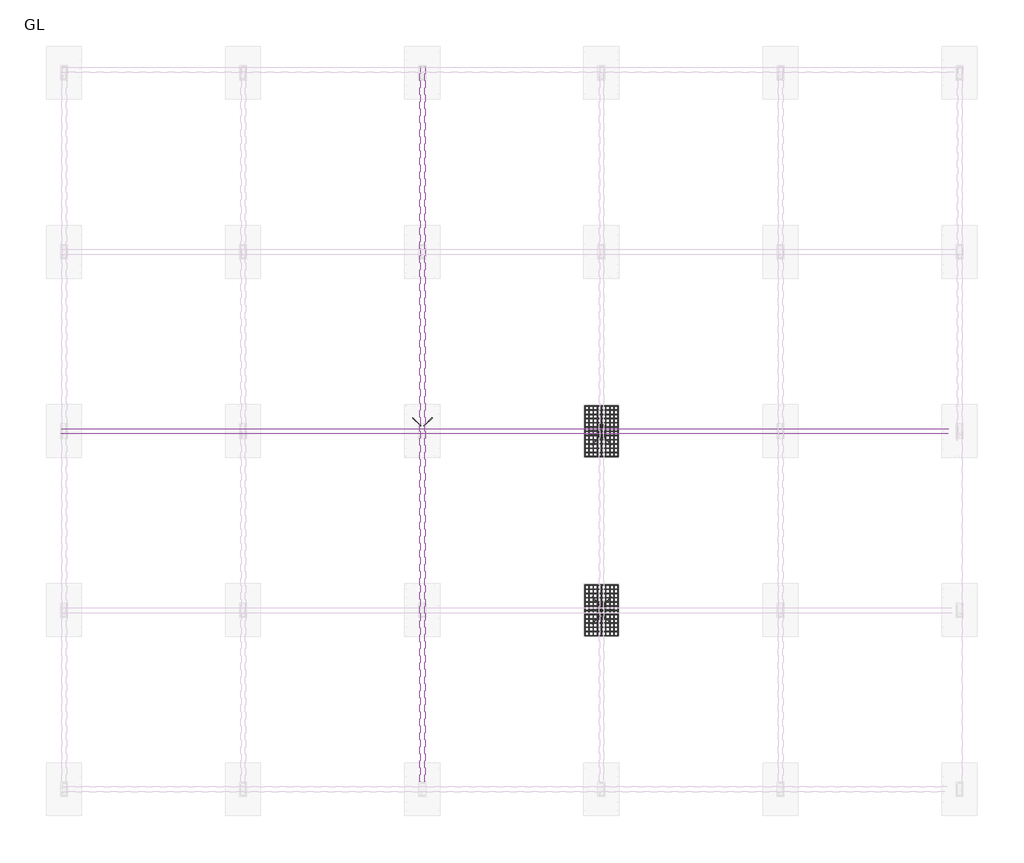
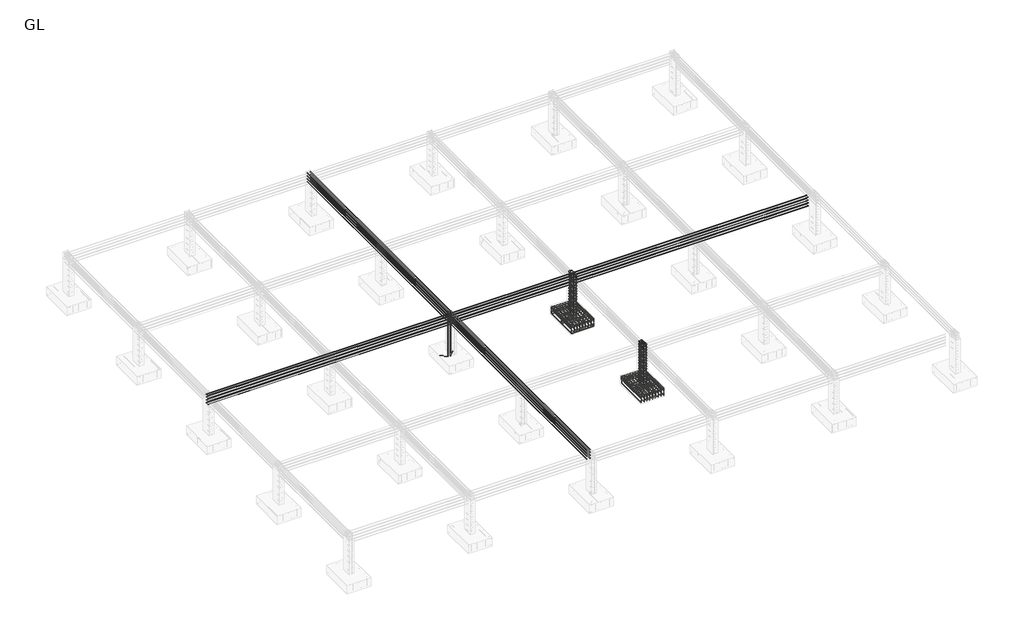
# One storey, part 8 of 16: 24 reinforcing bars.
"""IFC4 building model written with IfcOpenShell, lengths in millimetres."""

from ifc_helpers import new_model, si_unit, point, frame, origin, place, context, project, spatial, polyline, circle_curve, trimmed, segment, composite_curve, source, transform, mapped, element, save
from ifc_brep_helpers import swept_disk

model = new_model("IFC4")

# Units and contexts
model_context = context("Model", 3, world=origin())
ifc_project = project(units=[si_unit("LENGTHUNIT", "METRE", prefix="MILLI")], contexts=[model_context])

# Site, building, storey
site = spatial("IfcSite", under=ifc_project)
building = spatial("IfcBuilding", under=site)
storey = spatial("IfcBuildingStorey", under=building, Name="GL", Elevation=-1829.0)

# Reinforcing bars
placement = place(None, origin())
reinforcing_bar_shape = source(origin(), model_context, "Body", "SolidModel", [
    swept_disk(composite_curve([segment(polyline([(-3954.9544379, -7223.1167521, -2089.0), (-3954.9544379, -7223.1167521, -2213.0)]), True, "CONTINUOUS"), segment(trimmed(circle_curve(frame((-3984.9544379, -7223.1167521, -2213.0), z_axis=(0.0, 1.0, 0.0), x_axis=(30.0, 0.0, 0.0)), 30.0), [point((-3954.9544379, -7223.1167521, -2213.0))], [point((-3984.9544379, -7223.1167521, -2243.0))], True, "CARTESIAN"), True, "CONTINUOUS"), segment(polyline([(-3984.9544379, -7223.1167521, -2243.0), (-5052.9544379, -7223.1167521, -2243.0)]), True, "CONTINUOUS"), segment(trimmed(circle_curve(frame((-5052.9544379, -7223.1167521, -2213.0), z_axis=(0.0, 1.0, 0.0), x_axis=(0.0, 0.0, -30.0)), 30.0), [point((-5052.9544379, -7223.1167521, -2243.0))], [point((-5082.9544379, -7223.1167521, -2213.0))], True, "CARTESIAN"), True, "CONTINUOUS"), segment(polyline([(-5082.9544379, -7223.1167521, -2213.0), (-5082.9544379, -7223.1167521, -2089.0)]), True, "CONTINUOUS")], self_intersect=False), 6.0),
])
element("IfcReinforcingBar", 1, at=placement, inside=storey, context=model_context, shape_type="MappedRepresentation", body=[
    mapped(reinforcing_bar_shape, transform((0.0, 0.0, 0.0), x_axis=(1.0, 0.0, 0.0), y_axis=(0.0, 1.0, 0.0), z_axis=(0.0, 0.0, 1.0))),
    mapped(reinforcing_bar_shape, transform((0.0, -864.0, 0.0), x_axis=(1.0, 0.0, 0.0), y_axis=(0.0, 1.0, 0.0), z_axis=(0.0, 0.0, 1.0))),
    mapped(reinforcing_bar_shape, transform((0.0, -1728.0, 0.0), x_axis=(1.0, 0.0, 0.0), y_axis=(0.0, 1.0, 0.0), z_axis=(0.0, 0.0, 1.0))),
])
reinforcing_bar_2_shape = source(origin(), model_context, "Body", "SolidModel", [
    swept_disk(composite_curve([segment(polyline([(-5082.9544379, -7223.1167521, -2022.436678), (-5082.9544379, -7223.1167521, -1898.436678)]), True, "CONTINUOUS"), segment(trimmed(circle_curve(frame((-5052.9544379, -7223.1167521, -1898.436678), z_axis=(0.0, 1.0, 0.0), x_axis=(-30.0, 0.0, 0.0)), 30.0), [point((-5082.9544379, -7223.1167521, -1898.436678))], [point((-5052.9544379, -7223.1167521, -1868.436678))], True, "CARTESIAN"), True, "CONTINUOUS"), segment(polyline([(-5052.9544379, -7223.1167521, -1868.436678), (-3984.9544379, -7223.1167521, -1868.436678)]), True, "CONTINUOUS"), segment(trimmed(circle_curve(frame((-3984.9544379, -7223.1167521, -1898.436678), z_axis=(0.0, 1.0, 0.0), x_axis=(0.0, 0.0, 30.0)), 30.0), [point((-3984.9544379, -7223.1167521, -1868.436678))], [point((-3954.9544379, -7223.1167521, -1898.436678))], True, "CARTESIAN"), True, "CONTINUOUS"), segment(polyline([(-3954.9544379, -7223.1167521, -1898.436678), (-3954.9544379, -7223.1167521, -2022.436678)]), True, "CONTINUOUS")], self_intersect=False), 6.0),
])
element("IfcReinforcingBar", 2, at=placement, inside=storey, context=model_context, shape_type="MappedRepresentation", body=[
    mapped(reinforcing_bar_2_shape, transform((0.0, 0.0, 0.0), x_axis=(1.0, 0.0, 0.0), y_axis=(0.0, 1.0, 0.0), z_axis=(0.0, 0.0, 1.0))),
    mapped(reinforcing_bar_2_shape, transform((0.0, -144.0, 0.0), x_axis=(1.0, 0.0, 0.0), y_axis=(0.0, 1.0, 0.0), z_axis=(0.0, 0.0, 1.0))),
    mapped(reinforcing_bar_2_shape, transform((0.0, -288.0, 0.0), x_axis=(1.0, 0.0, 0.0), y_axis=(0.0, 1.0, 0.0), z_axis=(0.0, 0.0, 1.0))),
    mapped(reinforcing_bar_2_shape, transform((0.0, -432.0, 0.0), x_axis=(1.0, 0.0, 0.0), y_axis=(0.0, 1.0, 0.0), z_axis=(0.0, 0.0, 1.0))),
    mapped(reinforcing_bar_2_shape, transform((0.0, -576.0, 0.0), x_axis=(1.0, 0.0, 0.0), y_axis=(0.0, 1.0, 0.0), z_axis=(0.0, 0.0, 1.0))),
    mapped(reinforcing_bar_2_shape, transform((0.0, -720.0, 0.0), x_axis=(1.0, 0.0, 0.0), y_axis=(0.0, 1.0, 0.0), z_axis=(0.0, 0.0, 1.0))),
    mapped(reinforcing_bar_2_shape, transform((0.0, -864.0, 0.0), x_axis=(1.0, 0.0, 0.0), y_axis=(0.0, 1.0, 0.0), z_axis=(0.0, 0.0, 1.0))),
    mapped(reinforcing_bar_2_shape, transform((0.0, -1008.0, 0.0), x_axis=(1.0, 0.0, 0.0), y_axis=(0.0, 1.0, 0.0), z_axis=(0.0, 0.0, 1.0))),
    mapped(reinforcing_bar_2_shape, transform((0.0, -1152.0, 0.0), x_axis=(1.0, 0.0, 0.0), y_axis=(0.0, 1.0, 0.0), z_axis=(0.0, 0.0, 1.0))),
    mapped(reinforcing_bar_2_shape, transform((0.0, -1296.0, 0.0), x_axis=(1.0, 0.0, 0.0), y_axis=(0.0, 1.0, 0.0), z_axis=(0.0, 0.0, 1.0))),
    mapped(reinforcing_bar_2_shape, transform((0.0, -1440.0, 0.0), x_axis=(1.0, 0.0, 0.0), y_axis=(0.0, 1.0, 0.0), z_axis=(0.0, 0.0, 1.0))),
    mapped(reinforcing_bar_2_shape, transform((0.0, -1584.0, 0.0), x_axis=(1.0, 0.0, 0.0), y_axis=(0.0, 1.0, 0.0), z_axis=(0.0, 0.0, 1.0))),
    mapped(reinforcing_bar_2_shape, transform((0.0, -1728.0, 0.0), x_axis=(1.0, 0.0, 0.0), y_axis=(0.0, 1.0, 0.0), z_axis=(0.0, 0.0, 1.0))),
])
reinforcing_bar_3_shape = source(origin(), model_context, "Body", "SolidModel", [
    swept_disk(composite_curve([segment(polyline([(-5082.9544379, -8951.1167521, -2027.5081232), (-5082.9544379, -8951.1167521, -1903.5081232)]), True, "CONTINUOUS"), segment(trimmed(circle_curve(frame((-5082.9544379, -8921.1167521, -1903.5081232), z_axis=(-1.0, 0.0, 0.0), x_axis=(0.0, -30.0, 0.0)), 30.0), [point((-5082.9544379, -8951.1167521, -1903.5081232))], [point((-5082.9544379, -8921.1167521, -1873.5081232))], True, "CARTESIAN"), True, "CONTINUOUS"), segment(polyline([(-5082.9544379, -8921.1167521, -1873.5081232), (-5082.9544379, -7253.1167521, -1873.5081232)]), True, "CONTINUOUS"), segment(trimmed(circle_curve(frame((-5082.9544379, -7253.1167521, -1903.5081232), z_axis=(-1.0, 0.0, 0.0), x_axis=(0.0, 0.0, 30.0)), 30.0), [point((-5082.9544379, -7253.1167521, -1873.5081232))], [point((-5082.9544379, -7223.1167521, -1903.5081232))], True, "CARTESIAN"), True, "CONTINUOUS"), segment(polyline([(-5082.9544379, -7223.1167521, -1903.5081232), (-5082.9544379, -7223.1167521, -2027.5081232)]), True, "CONTINUOUS")], self_intersect=False), 6.0),
])
element("IfcReinforcingBar", 3, at=placement, inside=storey, context=model_context, shape_type="MappedRepresentation", body=[
    mapped(reinforcing_bar_3_shape, transform((0.0, 0.0, 0.0), x_axis=(1.0, 0.0, 0.0), y_axis=(0.0, 1.0, 0.0), z_axis=(0.0, 0.0, 1.0))),
    mapped(reinforcing_bar_3_shape, transform((141.0, 0.0, 0.0), x_axis=(1.0, 0.0, 0.0), y_axis=(0.0, 1.0, 0.0), z_axis=(0.0, 0.0, 1.0))),
    mapped(reinforcing_bar_3_shape, transform((282.0, 0.0, 0.0), x_axis=(1.0, 0.0, 0.0), y_axis=(0.0, 1.0, 0.0), z_axis=(0.0, 0.0, 1.0))),
    mapped(reinforcing_bar_3_shape, transform((423.0, 0.0, 0.0), x_axis=(1.0, 0.0, 0.0), y_axis=(0.0, 1.0, 0.0), z_axis=(0.0, 0.0, 1.0))),
    mapped(reinforcing_bar_3_shape, transform((564.0, 0.0, 0.0), x_axis=(1.0, 0.0, 0.0), y_axis=(0.0, 1.0, 0.0), z_axis=(0.0, 0.0, 1.0))),
    mapped(reinforcing_bar_3_shape, transform((705.0, 0.0, 0.0), x_axis=(1.0, 0.0, 0.0), y_axis=(0.0, 1.0, 0.0), z_axis=(0.0, 0.0, 1.0))),
    mapped(reinforcing_bar_3_shape, transform((846.0, 0.0, 0.0), x_axis=(1.0, 0.0, 0.0), y_axis=(0.0, 1.0, 0.0), z_axis=(0.0, 0.0, 1.0))),
    mapped(reinforcing_bar_3_shape, transform((987.0, 0.0, 0.0), x_axis=(1.0, 0.0, 0.0), y_axis=(0.0, 1.0, 0.0), z_axis=(0.0, 0.0, 1.0))),
    mapped(reinforcing_bar_3_shape, transform((1128.0, 0.0, 0.0), x_axis=(1.0, 0.0, 0.0), y_axis=(0.0, 1.0, 0.0), z_axis=(0.0, 0.0, 1.0))),
])
reinforcing_bar_4_shape = source(origin(), model_context, "Body", "SolidModel", [
    swept_disk(composite_curve([segment(polyline([(-3954.9544379, -8951.1167521, -2080.6239909), (-3954.9544379, -8951.1167521, -2204.6239909)]), True, "CONTINUOUS"), segment(trimmed(circle_curve(frame((-3954.9544379, -8921.1167521, -2204.6239909), z_axis=(1.0, 0.0, 0.0), x_axis=(0.0, -30.0, 0.0)), 30.0), [point((-3954.9544379, -8951.1167521, -2204.6239909))], [point((-3954.9544379, -8921.1167521, -2234.6239909))], True, "CARTESIAN"), True, "CONTINUOUS"), segment(polyline([(-3954.9544379, -8921.1167521, -2234.6239909), (-3954.9544379, -7266.1421892, -2234.6239909)]), True, "CONTINUOUS"), segment(trimmed(circle_curve(frame((-3954.9544379, -7266.1421892, -2204.6239909), z_axis=(1.0, 0.0, 0.0), x_axis=(0.0, 0.0, -30.0)), 30.0), [point((-3954.9544379, -7266.1421892, -2234.6239909))], [point((-3954.9544379, -7236.1421892, -2204.6239909))], True, "CARTESIAN"), True, "CONTINUOUS"), segment(polyline([(-3954.9544379, -7236.1421892, -2204.6239909), (-3954.9544379, -7236.1421892, -2080.6239909)]), True, "CONTINUOUS")], self_intersect=False), 6.0),
])
element("IfcReinforcingBar", 4, at=placement, inside=storey, context=model_context, shape_type="MappedRepresentation", body=[
    mapped(reinforcing_bar_4_shape, transform((0.0, 0.0, 0.0), x_axis=(1.0, 0.0, 0.0), y_axis=(0.0, 1.0, 0.0), z_axis=(0.0, 0.0, 1.0))),
    mapped(reinforcing_bar_4_shape, transform((-141.0, 0.0, 0.0), x_axis=(1.0, 0.0, 0.0), y_axis=(0.0, 1.0, 0.0), z_axis=(0.0, 0.0, 1.0))),
    mapped(reinforcing_bar_4_shape, transform((-282.0, 0.0, 0.0), x_axis=(1.0, 0.0, 0.0), y_axis=(0.0, 1.0, 0.0), z_axis=(0.0, 0.0, 1.0))),
    mapped(reinforcing_bar_4_shape, transform((-423.0, 0.0, 0.0), x_axis=(1.0, 0.0, 0.0), y_axis=(0.0, 1.0, 0.0), z_axis=(0.0, 0.0, 1.0))),
    mapped(reinforcing_bar_4_shape, transform((-564.0, 0.0, 0.0), x_axis=(1.0, 0.0, 0.0), y_axis=(0.0, 1.0, 0.0), z_axis=(0.0, 0.0, 1.0))),
    mapped(reinforcing_bar_4_shape, transform((-705.0, 0.0, 0.0), x_axis=(1.0, 0.0, 0.0), y_axis=(0.0, 1.0, 0.0), z_axis=(0.0, 0.0, 1.0))),
    mapped(reinforcing_bar_4_shape, transform((-846.0, 0.0, 0.0), x_axis=(1.0, 0.0, 0.0), y_axis=(0.0, 1.0, 0.0), z_axis=(0.0, 0.0, 1.0))),
    mapped(reinforcing_bar_4_shape, transform((-987.0, 0.0, 0.0), x_axis=(1.0, 0.0, 0.0), y_axis=(0.0, 1.0, 0.0), z_axis=(0.0, 0.0, 1.0))),
    mapped(reinforcing_bar_4_shape, transform((-1128.0, 0.0, 0.0), x_axis=(1.0, 0.0, 0.0), y_axis=(0.0, 1.0, 0.0), z_axis=(0.0, 0.0, 1.0))),
])
reinforcing_bar_5_shape = source(origin(), model_context, "Body", "SolidModel", [
    swept_disk(composite_curve([segment(polyline([(-5082.9544379, -13319.1167521, -2022.436678), (-5082.9544379, -13319.1167521, -1898.436678)]), True, "CONTINUOUS"), segment(trimmed(circle_curve(frame((-5052.9544379, -13319.1167521, -1898.436678), z_axis=(0.0, 1.0, 0.0), x_axis=(-30.0, 0.0, 0.0)), 30.0), [point((-5082.9544379, -13319.1167521, -1898.436678))], [point((-5052.9544379, -13319.1167521, -1868.436678))], True, "CARTESIAN"), True, "CONTINUOUS"), segment(polyline([(-5052.9544379, -13319.1167521, -1868.436678), (-3984.9544379, -13319.1167521, -1868.436678)]), True, "CONTINUOUS"), segment(trimmed(circle_curve(frame((-3984.9544379, -13319.1167521, -1898.436678), z_axis=(0.0, 1.0, 0.0), x_axis=(0.0, 0.0, 30.0)), 30.0), [point((-3984.9544379, -13319.1167521, -1868.436678))], [point((-3954.9544379, -13319.1167521, -1898.436678))], True, "CARTESIAN"), True, "CONTINUOUS"), segment(polyline([(-3954.9544379, -13319.1167521, -1898.436678), (-3954.9544379, -13319.1167521, -2022.436678)]), True, "CONTINUOUS")], self_intersect=False), 6.0),
])
element("IfcReinforcingBar", 5, at=placement, inside=storey, context=model_context, shape_type="MappedRepresentation", body=[
    mapped(reinforcing_bar_5_shape, transform((0.0, 0.0, 0.0), x_axis=(1.0, 0.0, 0.0), y_axis=(0.0, 1.0, 0.0), z_axis=(0.0, 0.0, 1.0))),
    mapped(reinforcing_bar_5_shape, transform((0.0, -144.0, 0.0), x_axis=(1.0, 0.0, 0.0), y_axis=(0.0, 1.0, 0.0), z_axis=(0.0, 0.0, 1.0))),
    mapped(reinforcing_bar_5_shape, transform((0.0, -288.0, 0.0), x_axis=(1.0, 0.0, 0.0), y_axis=(0.0, 1.0, 0.0), z_axis=(0.0, 0.0, 1.0))),
    mapped(reinforcing_bar_5_shape, transform((0.0, -432.0, 0.0), x_axis=(1.0, 0.0, 0.0), y_axis=(0.0, 1.0, 0.0), z_axis=(0.0, 0.0, 1.0))),
    mapped(reinforcing_bar_5_shape, transform((0.0, -576.0, 0.0), x_axis=(1.0, 0.0, 0.0), y_axis=(0.0, 1.0, 0.0), z_axis=(0.0, 0.0, 1.0))),
    mapped(reinforcing_bar_5_shape, transform((0.0, -720.0, 0.0), x_axis=(1.0, 0.0, 0.0), y_axis=(0.0, 1.0, 0.0), z_axis=(0.0, 0.0, 1.0))),
    mapped(reinforcing_bar_5_shape, transform((0.0, -864.0, 0.0), x_axis=(1.0, 0.0, 0.0), y_axis=(0.0, 1.0, 0.0), z_axis=(0.0, 0.0, 1.0))),
    mapped(reinforcing_bar_5_shape, transform((0.0, -1008.0, 0.0), x_axis=(1.0, 0.0, 0.0), y_axis=(0.0, 1.0, 0.0), z_axis=(0.0, 0.0, 1.0))),
    mapped(reinforcing_bar_5_shape, transform((0.0, -1152.0, 0.0), x_axis=(1.0, 0.0, 0.0), y_axis=(0.0, 1.0, 0.0), z_axis=(0.0, 0.0, 1.0))),
    mapped(reinforcing_bar_5_shape, transform((0.0, -1296.0, 0.0), x_axis=(1.0, 0.0, 0.0), y_axis=(0.0, 1.0, 0.0), z_axis=(0.0, 0.0, 1.0))),
    mapped(reinforcing_bar_5_shape, transform((0.0, -1440.0, 0.0), x_axis=(1.0, 0.0, 0.0), y_axis=(0.0, 1.0, 0.0), z_axis=(0.0, 0.0, 1.0))),
    mapped(reinforcing_bar_5_shape, transform((0.0, -1584.0, 0.0), x_axis=(1.0, 0.0, 0.0), y_axis=(0.0, 1.0, 0.0), z_axis=(0.0, 0.0, 1.0))),
    mapped(reinforcing_bar_5_shape, transform((0.0, -1728.0, 0.0), x_axis=(1.0, 0.0, 0.0), y_axis=(0.0, 1.0, 0.0), z_axis=(0.0, 0.0, 1.0))),
])
reinforcing_bar_6_shape = source(origin(), model_context, "Body", "SolidModel", [
    swept_disk(composite_curve([segment(polyline([(-5082.9544379, -15047.1167521, -2027.5081232), (-5082.9544379, -15047.1167521, -1903.5081232)]), True, "CONTINUOUS"), segment(trimmed(circle_curve(frame((-5082.9544379, -15017.1167521, -1903.5081232), z_axis=(-1.0, 0.0, 0.0), x_axis=(0.0, -30.0, 0.0)), 30.0), [point((-5082.9544379, -15047.1167521, -1903.5081232))], [point((-5082.9544379, -15017.1167521, -1873.5081232))], True, "CARTESIAN"), True, "CONTINUOUS"), segment(polyline([(-5082.9544379, -15017.1167521, -1873.5081232), (-5082.9544379, -13349.1167521, -1873.5081232)]), True, "CONTINUOUS"), segment(trimmed(circle_curve(frame((-5082.9544379, -13349.1167521, -1903.5081232), z_axis=(-1.0, 0.0, 0.0), x_axis=(0.0, 0.0, 30.0)), 30.0), [point((-5082.9544379, -13349.1167521, -1873.5081232))], [point((-5082.9544379, -13319.1167521, -1903.5081232))], True, "CARTESIAN"), True, "CONTINUOUS"), segment(polyline([(-5082.9544379, -13319.1167521, -1903.5081232), (-5082.9544379, -13319.1167521, -2027.5081232)]), True, "CONTINUOUS")], self_intersect=False), 6.0),
])
element("IfcReinforcingBar", 6, at=placement, inside=storey, context=model_context, shape_type="MappedRepresentation", body=[
    mapped(reinforcing_bar_6_shape, transform((0.0, 0.0, 0.0), x_axis=(1.0, 0.0, 0.0), y_axis=(0.0, 1.0, 0.0), z_axis=(0.0, 0.0, 1.0))),
    mapped(reinforcing_bar_6_shape, transform((141.0, 0.0, 0.0), x_axis=(1.0, 0.0, 0.0), y_axis=(0.0, 1.0, 0.0), z_axis=(0.0, 0.0, 1.0))),
    mapped(reinforcing_bar_6_shape, transform((282.0, 0.0, 0.0), x_axis=(1.0, 0.0, 0.0), y_axis=(0.0, 1.0, 0.0), z_axis=(0.0, 0.0, 1.0))),
    mapped(reinforcing_bar_6_shape, transform((423.0, 0.0, 0.0), x_axis=(1.0, 0.0, 0.0), y_axis=(0.0, 1.0, 0.0), z_axis=(0.0, 0.0, 1.0))),
    mapped(reinforcing_bar_6_shape, transform((564.0, 0.0, 0.0), x_axis=(1.0, 0.0, 0.0), y_axis=(0.0, 1.0, 0.0), z_axis=(0.0, 0.0, 1.0))),
    mapped(reinforcing_bar_6_shape, transform((705.0, 0.0, 0.0), x_axis=(1.0, 0.0, 0.0), y_axis=(0.0, 1.0, 0.0), z_axis=(0.0, 0.0, 1.0))),
    mapped(reinforcing_bar_6_shape, transform((846.0, 0.0, 0.0), x_axis=(1.0, 0.0, 0.0), y_axis=(0.0, 1.0, 0.0), z_axis=(0.0, 0.0, 1.0))),
    mapped(reinforcing_bar_6_shape, transform((987.0, 0.0, 0.0), x_axis=(1.0, 0.0, 0.0), y_axis=(0.0, 1.0, 0.0), z_axis=(0.0, 0.0, 1.0))),
    mapped(reinforcing_bar_6_shape, transform((1128.0, 0.0, 0.0), x_axis=(1.0, 0.0, 0.0), y_axis=(0.0, 1.0, 0.0), z_axis=(0.0, 0.0, 1.0))),
])
reinforcing_bar_7_shape = source(origin(), model_context, "Body", "SolidModel", [
    swept_disk(composite_curve([segment(polyline([(-3954.9544379, -15047.1167521, -2080.6239909), (-3954.9544379, -15047.1167521, -2204.6239909)]), True, "CONTINUOUS"), segment(trimmed(circle_curve(frame((-3954.9544379, -15017.1167521, -2204.6239909), z_axis=(1.0, 0.0, 0.0), x_axis=(0.0, -30.0, 0.0)), 30.0), [point((-3954.9544379, -15047.1167521, -2204.6239909))], [point((-3954.9544379, -15017.1167521, -2234.6239909))], True, "CARTESIAN"), True, "CONTINUOUS"), segment(polyline([(-3954.9544379, -15017.1167521, -2234.6239909), (-3954.9544379, -13362.1421892, -2234.6239909)]), True, "CONTINUOUS"), segment(trimmed(circle_curve(frame((-3954.9544379, -13362.1421892, -2204.6239909), z_axis=(1.0, 0.0, 0.0), x_axis=(0.0, 0.0, -30.0)), 30.0), [point((-3954.9544379, -13362.1421892, -2234.6239909))], [point((-3954.9544379, -13332.1421892, -2204.6239909))], True, "CARTESIAN"), True, "CONTINUOUS"), segment(polyline([(-3954.9544379, -13332.1421892, -2204.6239909), (-3954.9544379, -13332.1421892, -2080.6239909)]), True, "CONTINUOUS")], self_intersect=False), 6.0),
])
element("IfcReinforcingBar", 7, at=placement, inside=storey, context=model_context, shape_type="MappedRepresentation", body=[
    mapped(reinforcing_bar_7_shape, transform((0.0, 0.0, 0.0), x_axis=(1.0, 0.0, 0.0), y_axis=(0.0, 1.0, 0.0), z_axis=(0.0, 0.0, 1.0))),
    mapped(reinforcing_bar_7_shape, transform((-141.0, 0.0, 0.0), x_axis=(1.0, 0.0, 0.0), y_axis=(0.0, 1.0, 0.0), z_axis=(0.0, 0.0, 1.0))),
    mapped(reinforcing_bar_7_shape, transform((-282.0, 0.0, 0.0), x_axis=(1.0, 0.0, 0.0), y_axis=(0.0, 1.0, 0.0), z_axis=(0.0, 0.0, 1.0))),
    mapped(reinforcing_bar_7_shape, transform((-423.0, 0.0, 0.0), x_axis=(1.0, 0.0, 0.0), y_axis=(0.0, 1.0, 0.0), z_axis=(0.0, 0.0, 1.0))),
    mapped(reinforcing_bar_7_shape, transform((-564.0, 0.0, 0.0), x_axis=(1.0, 0.0, 0.0), y_axis=(0.0, 1.0, 0.0), z_axis=(0.0, 0.0, 1.0))),
    mapped(reinforcing_bar_7_shape, transform((-705.0, 0.0, 0.0), x_axis=(1.0, 0.0, 0.0), y_axis=(0.0, 1.0, 0.0), z_axis=(0.0, 0.0, 1.0))),
    mapped(reinforcing_bar_7_shape, transform((-846.0, 0.0, 0.0), x_axis=(1.0, 0.0, 0.0), y_axis=(0.0, 1.0, 0.0), z_axis=(0.0, 0.0, 1.0))),
    mapped(reinforcing_bar_7_shape, transform((-987.0, 0.0, 0.0), x_axis=(1.0, 0.0, 0.0), y_axis=(0.0, 1.0, 0.0), z_axis=(0.0, 0.0, 1.0))),
    mapped(reinforcing_bar_7_shape, transform((-1128.0, 0.0, 0.0), x_axis=(1.0, 0.0, 0.0), y_axis=(0.0, 1.0, 0.0), z_axis=(0.0, 0.0, 1.0))),
])
element("IfcReinforcingBar", 8, at=placement, inside=storey, context=model_context, shape_type="SolidModel", body=[
    swept_disk(composite_curve([segment(polyline([(-10672.0642232, -7902.1692603, 241.0), (-10672.0642232, -7902.1692603, -2129.0)]), True, "CONTINUOUS"), segment(trimmed(circle_curve(frame((-10693.2774266, -7880.9560568, -2129.0), z_axis=(0.7071067811865218, 0.7071067811865733, 0.0), x_axis=(21.213203400000566, -21.213203500000418, 0.0)), 30.0), [point((-10672.0642232, -7902.1692603, -2129.0))], [point((-10693.2774266, -7880.9560568, -2159.0))], True, "CARTESIAN"), True, "CONTINUOUS"), segment(polyline([(-10693.2774266, -7880.9560568, -2159.0), (-10940.7648, -7633.4686834, -2159.0)]), True, "CONTINUOUS")], self_intersect=False), 6.0),
])
element("IfcReinforcingBar", 9, at=placement, inside=storey, context=model_context, shape_type="SolidModel", body=[
    swept_disk(composite_curve([segment(polyline([(-10557.8446527, -7902.1692603, 241.0), (-10557.8446527, -7902.1692603, -2129.0)]), True, "CONTINUOUS"), segment(trimmed(circle_curve(frame((-10536.6314492, -7880.9560568, -2129.0), z_axis=(0.7071067811865157, -0.7071067811865794, 0.0), x_axis=(-21.21320349999951, -21.213203500000418, 0.0)), 30.0), [point((-10557.8446527, -7902.1692603, -2129.0))], [point((-10536.6314492, -7880.9560568, -2159.0))], True, "CARTESIAN"), True, "CONTINUOUS"), segment(polyline([(-10536.6314492, -7880.9560568, -2159.0), (-10289.1440758, -7633.4686834, -2159.0)]), True, "CONTINUOUS")], self_intersect=False), 6.0),
])
reinforcing_bar_8_shape = source(origin(), model_context, "Body", "SolidModel", [
    swept_disk(composite_curve([segment(polyline([(-4511.4864005, -8162.2223078, -1793.0), (-4599.1676414, -8249.9035486, -1793.0)]), True, "CONTINUOUS"), segment(trimmed(circle_curve(frame((-4577.9544379, -8271.1167521, -1793.0), z_axis=(0.0, 0.0, 1.0), x_axis=(-21.213203500000418, 21.213203500001327, 0.0)), 30.0), [point((-4599.1676414, -8249.9035486, -1793.0))], [point((-4577.9544379, -8301.1167521, -1793.0))], True, "CARTESIAN"), True, "CONTINUOUS"), segment(polyline([(-4577.9544379, -8301.1167521, -1793.0), (-4459.9544379, -8301.1167521, -1793.0)]), True, "CONTINUOUS"), segment(trimmed(circle_curve(frame((-4459.9544379, -8271.1167521, -1793.0), z_axis=(0.0, 0.0, 1.0), x_axis=(0.0, -30.0, 0.0)), 30.0), [point((-4459.9544379, -8301.1167521, -1793.0))], [point((-4429.9544379, -8271.1167521, -1793.0))], True, "CARTESIAN"), True, "CONTINUOUS"), segment(polyline([(-4429.9544379, -8271.1167521, -1793.0), (-4429.9544379, -7903.1167521, -1793.0)]), True, "CONTINUOUS"), segment(trimmed(circle_curve(frame((-4459.8864962, -7903.1167521, -1795.0178916), z_axis=(-0.06726305234213417, 0.0, 0.9977352764083365), x_axis=(29.93205829999988, 0.0, 2.0178915999999845)), 30.0), [point((-4429.9544379, -7903.1167521, -1793.0))], [point((-4459.8864962, -7873.1167521, -1795.0178916))], True, "CARTESIAN"), True, "CONTINUOUS"), segment(polyline([(-4459.8864962, -7873.1167521, -1795.0178916), (-4578.0223796, -7873.1167521, -1802.9821084)]), True, "CONTINUOUS"), segment(trimmed(circle_curve(frame((-4578.0223796, -7903.1167521, -1802.9821084), z_axis=(-0.06726305234213417, 0.0, 0.9977352764083365), x_axis=(0.0, 30.0, 0.0)), 30.0), [point((-4578.0223796, -7873.1167521, -1802.9821084))], [point((-4607.9544379, -7903.1167521, -1805.0))], True, "CARTESIAN"), True, "CONTINUOUS"), segment(polyline([(-4607.9544379, -7903.1167521, -1805.0), (-4607.9544379, -8271.1167521, -1805.0)]), True, "CONTINUOUS"), segment(trimmed(circle_curve(frame((-4577.9544379, -8271.1167521, -1805.0), z_axis=(0.0, 0.0, 1.0), x_axis=(-30.0, 0.0, 0.0)), 30.0), [point((-4607.9544379, -8271.1167521, -1805.0))], [point((-4556.7412345, -8292.3299555, -1805.0))], True, "CARTESIAN"), True, "CONTINUOUS"), segment(polyline([(-4556.7412345, -8292.3299555, -1805.0), (-4469.0599936, -8204.6487146, -1805.0)]), True, "CONTINUOUS")], self_intersect=False), 6.0),
])
element("IfcReinforcingBar", 10, at=placement, inside=storey, context=model_context, shape_type="MappedRepresentation", body=[
    mapped(reinforcing_bar_8_shape, transform((0.0, 0.0, 0.0), x_axis=(1.0, 0.0, 0.0), y_axis=(0.0, 1.0, 0.0), z_axis=(0.0, 0.0, 1.0))),
    mapped(reinforcing_bar_8_shape, transform((0.0, 0.0, 144.8571429), x_axis=(1.0, 0.0, 0.0), y_axis=(0.0, 1.0, 0.0), z_axis=(0.0, 0.0, 1.0))),
    mapped(reinforcing_bar_8_shape, transform((0.0, 0.0, 289.7142857), x_axis=(1.0, 0.0, 0.0), y_axis=(0.0, 1.0, 0.0), z_axis=(0.0, 0.0, 1.0))),
    mapped(reinforcing_bar_8_shape, transform((0.0, 0.0, 434.5714286), x_axis=(1.0, 0.0, 0.0), y_axis=(0.0, 1.0, 0.0), z_axis=(0.0, 0.0, 1.0))),
    mapped(reinforcing_bar_8_shape, transform((0.0, 0.0, 579.4285714), x_axis=(1.0, 0.0, 0.0), y_axis=(0.0, 1.0, 0.0), z_axis=(0.0, 0.0, 1.0))),
    mapped(reinforcing_bar_8_shape, transform((0.0, 0.0, 724.2857143), x_axis=(1.0, 0.0, 0.0), y_axis=(0.0, 1.0, 0.0), z_axis=(0.0, 0.0, 1.0))),
    mapped(reinforcing_bar_8_shape, transform((0.0, 0.0, 869.1428571), x_axis=(1.0, 0.0, 0.0), y_axis=(0.0, 1.0, 0.0), z_axis=(0.0, 0.0, 1.0))),
    mapped(reinforcing_bar_8_shape, transform((0.0, 0.0, 1014.0), x_axis=(1.0, 0.0, 0.0), y_axis=(0.0, 1.0, 0.0), z_axis=(0.0, 0.0, 1.0))),
    mapped(reinforcing_bar_8_shape, transform((0.0, 0.0, 1158.8571429), x_axis=(1.0, 0.0, 0.0), y_axis=(0.0, 1.0, 0.0), z_axis=(0.0, 0.0, 1.0))),
    mapped(reinforcing_bar_8_shape, transform((0.0, 0.0, 1303.7142857), x_axis=(1.0, 0.0, 0.0), y_axis=(0.0, 1.0, 0.0), z_axis=(0.0, 0.0, 1.0))),
    mapped(reinforcing_bar_8_shape, transform((0.0, 0.0, 1448.5714286), x_axis=(1.0, 0.0, 0.0), y_axis=(0.0, 1.0, 0.0), z_axis=(0.0, 0.0, 1.0))),
    mapped(reinforcing_bar_8_shape, transform((0.0, 0.0, 1593.4285714), x_axis=(1.0, 0.0, 0.0), y_axis=(0.0, 1.0, 0.0), z_axis=(0.0, 0.0, 1.0))),
    mapped(reinforcing_bar_8_shape, transform((0.0, 0.0, 1738.2857143), x_axis=(1.0, 0.0, 0.0), y_axis=(0.0, 1.0, 0.0), z_axis=(0.0, 0.0, 1.0))),
    mapped(reinforcing_bar_8_shape, transform((0.0, 0.0, 1883.1428571), x_axis=(1.0, 0.0, 0.0), y_axis=(0.0, 1.0, 0.0), z_axis=(0.0, 0.0, 1.0))),
    mapped(reinforcing_bar_8_shape, transform((0.0, 0.0, 2028.0), x_axis=(1.0, 0.0, 0.0), y_axis=(0.0, 1.0, 0.0), z_axis=(0.0, 0.0, 1.0))),
])
element("IfcReinforcingBar", 11, at=placement, inside=storey, context=model_context, shape_type="SolidModel", body=[
    swept_disk(composite_curve([segment(polyline([(-4576.0642232, -8272.0642439, 241.0), (-4576.0642232, -8272.0642439, -2129.0)]), True, "CONTINUOUS"), segment(trimmed(circle_curve(frame((-4597.2774266, -8293.2774473, -2129.0), z_axis=(-0.7071067811865187, 0.7071067811865764, 0.0), x_axis=(21.213203399999657, 21.213203400000566, 0.0)), 30.0), [point((-4576.0642232, -8272.0642439, -2129.0))], [point((-4597.2774266, -8293.2774473, -2159.0))], True, "CARTESIAN"), True, "CONTINUOUS"), segment(polyline([(-4597.2774266, -8293.2774473, -2159.0), (-4844.7648, -8540.7648207, -2159.0)]), True, "CONTINUOUS")], self_intersect=False), 6.0),
])
element("IfcReinforcingBar", 12, at=placement, inside=storey, context=model_context, shape_type="SolidModel", body=[
    swept_disk(composite_curve([segment(polyline([(-4461.8446527, -8272.0642439, 241.0), (-4461.8446527, -8272.0642439, -2129.0)]), True, "CONTINUOUS"), segment(trimmed(circle_curve(frame((-4440.6314492, -8293.2774473, -2129.0), z_axis=(-0.7071067811865248, -0.7071067811865703, 0.0), x_axis=(-21.21320349999951, 21.213203400000566, 0.0)), 30.0), [point((-4461.8446527, -8272.0642439, -2129.0))], [point((-4440.6314492, -8293.2774473, -2159.0))], True, "CARTESIAN"), True, "CONTINUOUS"), segment(polyline([(-4440.6314492, -8293.2774473, -2159.0), (-4193.1440758, -8540.7648207, -2159.0)]), True, "CONTINUOUS")], self_intersect=False), 6.0),
])
reinforcing_bar_9_shape = source(origin(), model_context, "Body", "SolidModel", [
    swept_disk(composite_curve([segment(polyline([(-4576.0642232, -8194.9117405, 241.0), (-4576.0642232, -8194.9117405, -2129.0)]), True, "CONTINUOUS"), segment(trimmed(circle_curve(frame((-4606.0642232, -8194.9117405, -2129.0), z_axis=(0.0, 1.0, 0.0), x_axis=(30.0, 0.0, 0.0)), 30.0), [point((-4576.0642232, -8194.9117405, -2129.0))], [point((-4606.0642232, -8194.9117405, -2159.0))], True, "CARTESIAN"), True, "CONTINUOUS"), segment(polyline([(-4606.0642232, -8194.9117405, -2159.0), (-4956.0642232, -8194.9117405, -2159.0)]), True, "CONTINUOUS")], self_intersect=False), 6.0),
])
element("IfcReinforcingBar", 13, at=placement, inside=storey, context=model_context, shape_type="MappedRepresentation", body=[
    mapped(reinforcing_bar_9_shape, transform((0.0, 0.0, 0.0), x_axis=(1.0, 0.0, 0.0), y_axis=(0.0, 1.0, 0.0), z_axis=(0.0, 0.0, 1.0))),
    mapped(reinforcing_bar_9_shape, transform((0.0, 123.5823926, 0.0), x_axis=(1.0, 0.0, 0.0), y_axis=(0.0, 1.0, 0.0), z_axis=(0.0, 0.0, 1.0))),
    mapped(reinforcing_bar_9_shape, transform((0.0, 247.1647853, 0.0), x_axis=(1.0, 0.0, 0.0), y_axis=(0.0, 1.0, 0.0), z_axis=(0.0, 0.0, 1.0))),
])
reinforcing_bar_10_shape = source(origin(), model_context, "Body", "SolidModel", [
    swept_disk(composite_curve([segment(polyline([(-4511.4864005, -14258.2223078, -1793.0), (-4599.1676414, -14345.9035486, -1793.0)]), True, "CONTINUOUS"), segment(trimmed(circle_curve(frame((-4577.9544379, -14367.1167521, -1793.0), z_axis=(0.0, 0.0, 1.0), x_axis=(-21.213203500000418, 21.213203500001327, 0.0)), 30.0), [point((-4599.1676414, -14345.9035486, -1793.0))], [point((-4577.9544379, -14397.1167521, -1793.0))], True, "CARTESIAN"), True, "CONTINUOUS"), segment(polyline([(-4577.9544379, -14397.1167521, -1793.0), (-4459.9544379, -14397.1167521, -1793.0)]), True, "CONTINUOUS"), segment(trimmed(circle_curve(frame((-4459.9544379, -14367.1167521, -1793.0), z_axis=(0.0, 0.0, 1.0), x_axis=(0.0, -30.0, 0.0)), 30.0), [point((-4459.9544379, -14397.1167521, -1793.0))], [point((-4429.9544379, -14367.1167521, -1793.0))], True, "CARTESIAN"), True, "CONTINUOUS"), segment(polyline([(-4429.9544379, -14367.1167521, -1793.0), (-4429.9544379, -13999.1167521, -1793.0)]), True, "CONTINUOUS"), segment(trimmed(circle_curve(frame((-4459.8864962, -13999.1167521, -1795.0178916), z_axis=(-0.06726305234213417, 0.0, 0.9977352764083365), x_axis=(29.93205829999988, 0.0, 2.0178915999999845)), 30.0), [point((-4429.9544379, -13999.1167521, -1793.0))], [point((-4459.8864962, -13969.1167521, -1795.0178916))], True, "CARTESIAN"), True, "CONTINUOUS"), segment(polyline([(-4459.8864962, -13969.1167521, -1795.0178916), (-4578.0223796, -13969.1167521, -1802.9821084)]), True, "CONTINUOUS"), segment(trimmed(circle_curve(frame((-4578.0223796, -13999.1167521, -1802.9821084), z_axis=(-0.06726305234213417, 0.0, 0.9977352764083365), x_axis=(0.0, 30.0, 0.0)), 30.0), [point((-4578.0223796, -13969.1167521, -1802.9821084))], [point((-4607.9544379, -13999.1167521, -1805.0))], True, "CARTESIAN"), True, "CONTINUOUS"), segment(polyline([(-4607.9544379, -13999.1167521, -1805.0), (-4607.9544379, -14367.1167521, -1805.0)]), True, "CONTINUOUS"), segment(trimmed(circle_curve(frame((-4577.9544379, -14367.1167521, -1805.0), z_axis=(0.0, 0.0, 1.0), x_axis=(-30.0, 0.0, 0.0)), 30.0), [point((-4607.9544379, -14367.1167521, -1805.0))], [point((-4556.7412345, -14388.3299555, -1805.0))], True, "CARTESIAN"), True, "CONTINUOUS"), segment(polyline([(-4556.7412345, -14388.3299555, -1805.0), (-4469.0599936, -14300.6487146, -1805.0)]), True, "CONTINUOUS")], self_intersect=False), 6.0),
])
element("IfcReinforcingBar", 14, at=placement, inside=storey, context=model_context, shape_type="MappedRepresentation", body=[
    mapped(reinforcing_bar_10_shape, transform((0.0, 0.0, 0.0), x_axis=(1.0, 0.0, 0.0), y_axis=(0.0, 1.0, 0.0), z_axis=(0.0, 0.0, 1.0))),
    mapped(reinforcing_bar_10_shape, transform((0.0, 0.0, 144.8571429), x_axis=(1.0, 0.0, 0.0), y_axis=(0.0, 1.0, 0.0), z_axis=(0.0, 0.0, 1.0))),
    mapped(reinforcing_bar_10_shape, transform((0.0, 0.0, 289.7142857), x_axis=(1.0, 0.0, 0.0), y_axis=(0.0, 1.0, 0.0), z_axis=(0.0, 0.0, 1.0))),
    mapped(reinforcing_bar_10_shape, transform((0.0, 0.0, 434.5714286), x_axis=(1.0, 0.0, 0.0), y_axis=(0.0, 1.0, 0.0), z_axis=(0.0, 0.0, 1.0))),
    mapped(reinforcing_bar_10_shape, transform((0.0, 0.0, 579.4285714), x_axis=(1.0, 0.0, 0.0), y_axis=(0.0, 1.0, 0.0), z_axis=(0.0, 0.0, 1.0))),
    mapped(reinforcing_bar_10_shape, transform((0.0, 0.0, 724.2857143), x_axis=(1.0, 0.0, 0.0), y_axis=(0.0, 1.0, 0.0), z_axis=(0.0, 0.0, 1.0))),
    mapped(reinforcing_bar_10_shape, transform((0.0, 0.0, 869.1428571), x_axis=(1.0, 0.0, 0.0), y_axis=(0.0, 1.0, 0.0), z_axis=(0.0, 0.0, 1.0))),
    mapped(reinforcing_bar_10_shape, transform((0.0, 0.0, 1014.0), x_axis=(1.0, 0.0, 0.0), y_axis=(0.0, 1.0, 0.0), z_axis=(0.0, 0.0, 1.0))),
    mapped(reinforcing_bar_10_shape, transform((0.0, 0.0, 1158.8571429), x_axis=(1.0, 0.0, 0.0), y_axis=(0.0, 1.0, 0.0), z_axis=(0.0, 0.0, 1.0))),
    mapped(reinforcing_bar_10_shape, transform((0.0, 0.0, 1303.7142857), x_axis=(1.0, 0.0, 0.0), y_axis=(0.0, 1.0, 0.0), z_axis=(0.0, 0.0, 1.0))),
    mapped(reinforcing_bar_10_shape, transform((0.0, 0.0, 1448.5714286), x_axis=(1.0, 0.0, 0.0), y_axis=(0.0, 1.0, 0.0), z_axis=(0.0, 0.0, 1.0))),
    mapped(reinforcing_bar_10_shape, transform((0.0, 0.0, 1593.4285714), x_axis=(1.0, 0.0, 0.0), y_axis=(0.0, 1.0, 0.0), z_axis=(0.0, 0.0, 1.0))),
    mapped(reinforcing_bar_10_shape, transform((0.0, 0.0, 1738.2857143), x_axis=(1.0, 0.0, 0.0), y_axis=(0.0, 1.0, 0.0), z_axis=(0.0, 0.0, 1.0))),
    mapped(reinforcing_bar_10_shape, transform((0.0, 0.0, 1883.1428571), x_axis=(1.0, 0.0, 0.0), y_axis=(0.0, 1.0, 0.0), z_axis=(0.0, 0.0, 1.0))),
    mapped(reinforcing_bar_10_shape, transform((0.0, 0.0, 2028.0), x_axis=(1.0, 0.0, 0.0), y_axis=(0.0, 1.0, 0.0), z_axis=(0.0, 0.0, 1.0))),
])
element("IfcReinforcingBar", 15, at=placement, inside=storey, context=model_context, shape_type="SolidModel", body=[
    swept_disk(composite_curve([segment(polyline([(-4576.0642232, -14368.0642439, 241.0), (-4576.0642232, -14368.0642439, -2129.0)]), True, "CONTINUOUS"), segment(trimmed(circle_curve(frame((-4597.2774266, -14389.2774473, -2129.0), z_axis=(-0.7071067811865187, 0.7071067811865764, 0.0), x_axis=(21.213203399999657, 21.213203400000566, 0.0)), 30.0), [point((-4576.0642232, -14368.0642439, -2129.0))], [point((-4597.2774266, -14389.2774473, -2159.0))], True, "CARTESIAN"), True, "CONTINUOUS"), segment(polyline([(-4597.2774266, -14389.2774473, -2159.0), (-4844.7648, -14636.7648207, -2159.0)]), True, "CONTINUOUS")], self_intersect=False), 6.0),
])
element("IfcReinforcingBar", 16, at=placement, inside=storey, context=model_context, shape_type="SolidModel", body=[
    swept_disk(composite_curve([segment(polyline([(-4576.0642232, -13998.1692603, 241.0), (-4576.0642232, -13998.1692603, -2129.0)]), True, "CONTINUOUS"), segment(trimmed(circle_curve(frame((-4597.2774266, -13976.9560568, -2129.0), z_axis=(0.7071067811865218, 0.7071067811865733, 0.0), x_axis=(21.213203399999657, -21.21320349999951, 0.0)), 30.0), [point((-4576.0642232, -13998.1692603, -2129.0))], [point((-4597.2774266, -13976.9560568, -2159.0))], True, "CARTESIAN"), True, "CONTINUOUS"), segment(polyline([(-4597.2774266, -13976.9560568, -2159.0), (-4844.7648, -13729.4686834, -2159.0)]), True, "CONTINUOUS")], self_intersect=False), 6.0),
])
element("IfcReinforcingBar", 17, at=placement, inside=storey, context=model_context, shape_type="SolidModel", body=[
    swept_disk(composite_curve([segment(polyline([(-4461.8446527, -14368.0642439, 241.0), (-4461.8446527, -14368.0642439, -2129.0)]), True, "CONTINUOUS"), segment(trimmed(circle_curve(frame((-4440.6314492, -14389.2774473, -2129.0), z_axis=(-0.7071067811865248, -0.7071067811865703, 0.0), x_axis=(-21.21320349999951, 21.213203400000566, 0.0)), 30.0), [point((-4461.8446527, -14368.0642439, -2129.0))], [point((-4440.6314492, -14389.2774473, -2159.0))], True, "CARTESIAN"), True, "CONTINUOUS"), segment(polyline([(-4440.6314492, -14389.2774473, -2159.0), (-4193.1440758, -14636.7648207, -2159.0)]), True, "CONTINUOUS")], self_intersect=False), 6.0),
])
element("IfcReinforcingBar", 18, at=placement, inside=storey, context=model_context, shape_type="SolidModel", body=[
    swept_disk(composite_curve([segment(polyline([(-4461.8446527, -13998.1692603, 241.0), (-4461.8446527, -13998.1692603, -2129.0)]), True, "CONTINUOUS"), segment(trimmed(circle_curve(frame((-4440.6314492, -13976.9560568, -2129.0), z_axis=(0.7071067811865157, -0.7071067811865794, 0.0), x_axis=(-21.21320349999951, -21.21320349999951, 0.0)), 30.0), [point((-4461.8446527, -13998.1692603, -2129.0))], [point((-4440.6314492, -13976.9560568, -2159.0))], True, "CARTESIAN"), True, "CONTINUOUS"), segment(polyline([(-4440.6314492, -13976.9560568, -2159.0), (-4193.1440758, -13729.4686834, -2159.0)]), True, "CONTINUOUS")], self_intersect=False), 6.0),
])
reinforcing_bar_11_shape = source(origin(), model_context, "Body", "SolidModel", [
    swept_disk(composite_curve([segment(polyline([(-4576.0642232, -14290.9117405, 241.0), (-4576.0642232, -14290.9117405, -2129.0)]), True, "CONTINUOUS"), segment(trimmed(circle_curve(frame((-4606.0642232, -14290.9117405, -2129.0), z_axis=(0.0, 1.0, 0.0), x_axis=(30.0, 0.0, 0.0)), 30.0), [point((-4576.0642232, -14290.9117405, -2129.0))], [point((-4606.0642232, -14290.9117405, -2159.0))], True, "CARTESIAN"), True, "CONTINUOUS"), segment(polyline([(-4606.0642232, -14290.9117405, -2159.0), (-4956.0642232, -14290.9117405, -2159.0)]), True, "CONTINUOUS")], self_intersect=False), 6.0),
])
element("IfcReinforcingBar", 19, at=placement, inside=storey, context=model_context, shape_type="MappedRepresentation", body=[
    mapped(reinforcing_bar_11_shape, transform((0.0, 0.0, 0.0), x_axis=(1.0, 0.0, 0.0), y_axis=(0.0, 1.0, 0.0), z_axis=(0.0, 0.0, 1.0))),
    mapped(reinforcing_bar_11_shape, transform((0.0, 123.5823926, 0.0), x_axis=(1.0, 0.0, 0.0), y_axis=(0.0, 1.0, 0.0), z_axis=(0.0, 0.0, 1.0))),
    mapped(reinforcing_bar_11_shape, transform((0.0, 247.1647853, 0.0), x_axis=(1.0, 0.0, 0.0), y_axis=(0.0, 1.0, 0.0), z_axis=(0.0, 0.0, 1.0))),
])
reinforcing_bar_12_shape = source(origin(), model_context, "Body", "SolidModel", [
    swept_disk(composite_curve([segment(polyline([(-4461.8446527, -14290.9117405, 241.0), (-4461.8446527, -14290.9117405, -2129.0)]), True, "CONTINUOUS"), segment(trimmed(circle_curve(frame((-4431.8446527, -14290.9117405, -2129.0), z_axis=(0.0, -1.0, 0.0), x_axis=(-30.0, 0.0, 0.0)), 30.0), [point((-4461.8446527, -14290.9117405, -2129.0))], [point((-4431.8446527, -14290.9117405, -2159.0))], True, "CARTESIAN"), True, "CONTINUOUS"), segment(polyline([(-4431.8446527, -14290.9117405, -2159.0), (-4081.8446527, -14290.9117405, -2159.0)]), True, "CONTINUOUS")], self_intersect=False), 6.0),
])
element("IfcReinforcingBar", 20, at=placement, inside=storey, context=model_context, shape_type="MappedRepresentation", body=[
    mapped(reinforcing_bar_12_shape, transform((0.0, 0.0, 0.0), x_axis=(1.0, 0.0, 0.0), y_axis=(0.0, 1.0, 0.0), z_axis=(0.0, 0.0, 1.0))),
    mapped(reinforcing_bar_12_shape, transform((0.0, 123.5823926, 0.0), x_axis=(1.0, 0.0, 0.0), y_axis=(0.0, 1.0, 0.0), z_axis=(0.0, 0.0, 1.0))),
    mapped(reinforcing_bar_12_shape, transform((0.0, 247.1647853, 0.0), x_axis=(1.0, 0.0, 0.0), y_axis=(0.0, 1.0, 0.0), z_axis=(0.0, 0.0, 1.0))),
])
reinforcing_bar_13_shape = source(origin(), model_context, "Body", "SolidModel", [
    swept_disk(composite_curve([segment(polyline([(7287.2221744, -8015.8446741, 202.0203396), (-22901.9544379, -8015.8446741, 202.0203396)]), True, "CONTINUOUS")], self_intersect=False), 6.0),
])
element("IfcReinforcingBar", 21, at=placement, inside=storey, context=model_context, shape_type="MappedRepresentation", body=[
    mapped(reinforcing_bar_13_shape, transform((0.0, 0.0, 0.0), x_axis=(1.0, 0.0, 0.0), y_axis=(0.0, 1.0, 0.0), z_axis=(0.0, 0.0, 1.0))),
    mapped(reinforcing_bar_13_shape, transform((0.0, 0.0, -154.4227336), x_axis=(1.0, 0.0, 0.0), y_axis=(0.0, 1.0, 0.0), z_axis=(0.0, 0.0, 1.0))),
    mapped(reinforcing_bar_13_shape, transform((0.0, 0.0, -308.8454671), x_axis=(1.0, 0.0, 0.0), y_axis=(0.0, 1.0, 0.0), z_axis=(0.0, 0.0, 1.0))),
    mapped(reinforcing_bar_13_shape, transform((0.0, 0.0, -463.2682007), x_axis=(1.0, 0.0, 0.0), y_axis=(0.0, 1.0, 0.0), z_axis=(0.0, 0.0, 1.0))),
])
reinforcing_bar_14_shape = source(origin(), model_context, "Body", "SolidModel", [
    swept_disk(composite_curve([segment(polyline([(7276.3761049, -8166.5001023, -261.2478611), (-22901.9544379, -8166.5001023, -261.2478611)]), True, "CONTINUOUS")], self_intersect=False), 6.0),
])
element("IfcReinforcingBar", 22, at=placement, inside=storey, context=model_context, shape_type="MappedRepresentation", body=[
    mapped(reinforcing_bar_14_shape, transform((0.0, 0.0, 0.0), x_axis=(1.0, 0.0, 0.0), y_axis=(0.0, 1.0, 0.0), z_axis=(0.0, 0.0, 1.0))),
    mapped(reinforcing_bar_14_shape, transform((0.0, 0.0, 154.4227336), x_axis=(1.0, 0.0, 0.0), y_axis=(0.0, 1.0, 0.0), z_axis=(0.0, 0.0, 1.0))),
    mapped(reinforcing_bar_14_shape, transform((0.0, 0.0, 308.8454671), x_axis=(1.0, 0.0, 0.0), y_axis=(0.0, 1.0, 0.0), z_axis=(0.0, 0.0, 1.0))),
    mapped(reinforcing_bar_14_shape, transform((0.0, 0.0, 463.2682007), x_axis=(1.0, 0.0, 0.0), y_axis=(0.0, 1.0, 0.0), z_axis=(0.0, 0.0, 1.0))),
])
reinforcing_bar_15_shape = source(origin(), model_context, "Body", "SolidModel", [
    swept_disk(composite_curve([segment(polyline([(-10698.9544379, 4324.8832479, 205.9406865), (-10698.9544379, -20016.9253077, 205.9406865)]), True, "CONTINUOUS")], self_intersect=False), 6.0),
])
element("IfcReinforcingBar", 23, at=placement, inside=storey, context=model_context, shape_type="MappedRepresentation", body=[
    mapped(reinforcing_bar_15_shape, transform((0.0, 0.0, 0.0), x_axis=(1.0, 0.0, 0.0), y_axis=(0.0, 1.0, 0.0), z_axis=(0.0, 0.0, 1.0))),
    mapped(reinforcing_bar_15_shape, transform((0.0, 0.0, -154.6703549), x_axis=(1.0, 0.0, 0.0), y_axis=(0.0, 1.0, 0.0), z_axis=(0.0, 0.0, 1.0))),
    mapped(reinforcing_bar_15_shape, transform((0.0, 0.0, -309.3407097), x_axis=(1.0, 0.0, 0.0), y_axis=(0.0, 1.0, 0.0), z_axis=(0.0, 0.0, 1.0))),
    mapped(reinforcing_bar_15_shape, transform((0.0, 0.0, -464.0110646), x_axis=(1.0, 0.0, 0.0), y_axis=(0.0, 1.0, 0.0), z_axis=(0.0, 0.0, 1.0))),
])
reinforcing_bar_16_shape = source(origin(), model_context, "Body", "SolidModel", [
    swept_disk(composite_curve([segment(polyline([(-10530.9544379, 4324.8832479, -258.0703781), (-10530.9544379, -20012.8026881, -258.0703781)]), True, "CONTINUOUS")], self_intersect=False), 6.0),
])
element("IfcReinforcingBar", 24, at=placement, inside=storey, context=model_context, shape_type="MappedRepresentation", body=[
    mapped(reinforcing_bar_16_shape, transform((0.0, 0.0, 0.0), x_axis=(1.0, 0.0, 0.0), y_axis=(0.0, 1.0, 0.0), z_axis=(0.0, 0.0, 1.0))),
    mapped(reinforcing_bar_16_shape, transform((0.0, 0.0, 154.6703549), x_axis=(1.0, 0.0, 0.0), y_axis=(0.0, 1.0, 0.0), z_axis=(0.0, 0.0, 1.0))),
    mapped(reinforcing_bar_16_shape, transform((0.0, 0.0, 309.3407097), x_axis=(1.0, 0.0, 0.0), y_axis=(0.0, 1.0, 0.0), z_axis=(0.0, 0.0, 1.0))),
    mapped(reinforcing_bar_16_shape, transform((0.0, 0.0, 464.0110646), x_axis=(1.0, 0.0, 0.0), y_axis=(0.0, 1.0, 0.0), z_axis=(0.0, 0.0, 1.0))),
])

save(model, "model.ifc")

# Revit data of these elements
# Elements 1, 2, 3, 4, 5, 6, 7, 8, 9, 10, 11, 12, 13, 14, 15, 16, 17, 18, 19, 20, 21, 22, 23, 24 (IfcReinforcingBar)
#   Phase Created = New Construction
